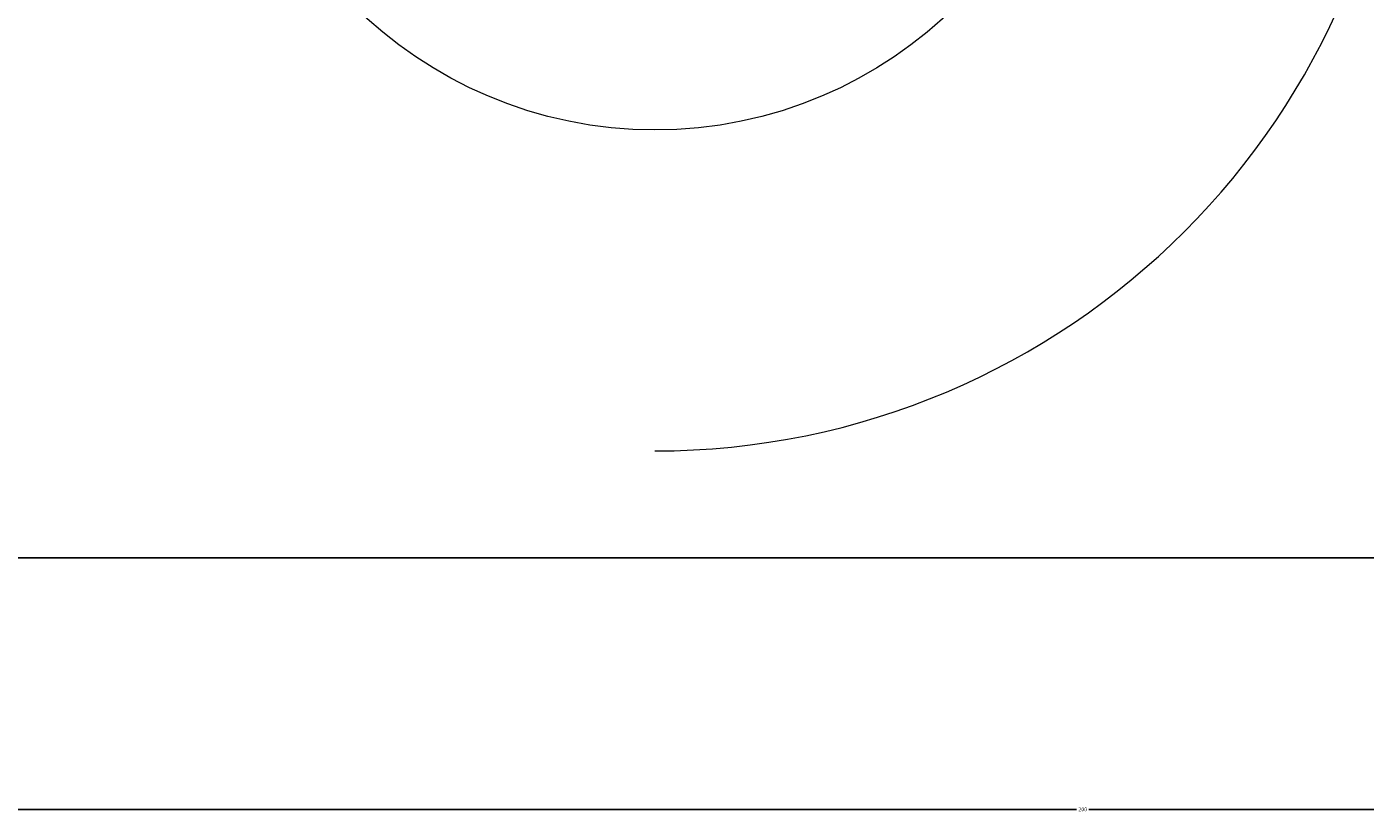
# Model space of a CAD drawing. Units: millimetres. Extents: x 3108 to 3332, y 1482 to 1586.
# Tile 2 of 5: x 3171 to 3233, y 1482 to 1519. Entities that reach past the tile are written whole.
import ezdxf

# ---------------------------------------------------------------- set-up
doc = ezdxf.new("R2010")
doc.units = ezdxf.units.MM
doc.layers.add('M-CONS', color=8, linetype='Continuous', lineweight=18)
doc.layers.add('M-DIMS', color=2, linetype='Continuous', lineweight=18)
doc.styles.get("Standard").update_dxf_attribs({"font": 'arial.ttf'})
doc.dimstyles.get("Standard").update_dxf_attribs({"dimtxt": 0.18, "dimasz": 0.18, "dimexe": 0.18, "dimexo": 0.0625, "dimgap": 0.09, "dimtad": 0, "dimtih": 1, "dimtoh": 1, "dimdec": 4, "dimzin": 0, "dimdsep": 46, "dimtxsty": 'Standard', "dimcen": 0.09, "dimadec": 0, "dimazin": 0, "dimtfac": 1, "dimtdec": 4, "dimtofl": 0, "dimtmove": 0, "dimatfit": 3, "dimfxl": 1, "dimtolj": 1, "dimtzin": 0, "dimarcsym": 0})

# ---------------------------------------------------------------- blocks, each defined once
blk = doc.blocks.new('*D1')
at = {"layer": 'Defpoints', "color": 0, "transparency": 16777216}
for p in [(3119.945, 1498.943), (3319.945, 1493.943), (3319.945, 1482.193)]:
    blk.add_point(p, dxfattribs=at)
at = {"layer": 'M-DIMS', "color": 0, "lineweight": -2, "transparency": 16777216}
for p, q in [((3119.945, 1498.881), (3119.945, 1482.013)), ((3319.945, 1493.881), (3319.945, 1482.013)), ((3120.125, 1482.193), (3219.655, 1482.193)), ((3319.765, 1482.193), (3220.235, 1482.193))]:
    blk.add_line(p, q, dxfattribs=at)
at = {"layer": 'M-DIMS', "color": 0, "transparency": 16777216}
for points in [[(3120.125, 1482.223), (3120.125, 1482.163), (3119.945, 1482.193)], [(3319.765, 1482.223), (3319.765, 1482.163), (3319.945, 1482.193)]]:
    blk.add_solid(points, dxfattribs=at)
at = {"layer": 'M-DIMS', "color": 0, "transparency": 16777216, "insert": (3219.945, 1482.193), "char_height": 0.18, "attachment_point": 5}
blk.add_mtext('\\A1;200', dxfattribs=at)
blk = doc.blocks.new('*D9')
at = {"layer": 'Defpoints', "color": 0, "transparency": 16777216}
for p in [(3108.195, 1533.943), (3199.945, 1533.943), (3159.945, 1498.943)]:
    blk.add_point(p, dxfattribs=at)
at = {"layer": 'M-DIMS', "color": 0, "lineweight": -2, "transparency": 16777216}
for p, q in [((3199.882, 1533.943), (3108.015, 1533.943)), ((3108.195, 1533.763), (3108.195, 1516.625)), ((3108.195, 1499.123), (3108.195, 1516.261)), ((3159.882, 1498.943), (3108.015, 1498.943))]:
    blk.add_line(p, q, dxfattribs=at)
at = {"layer": 'M-DIMS', "color": 0, "transparency": 16777216}
for points in [[(3108.165, 1533.763), (3108.225, 1533.763), (3108.195, 1533.943)], [(3108.165, 1499.123), (3108.225, 1499.123), (3108.195, 1498.943)]]:
    blk.add_solid(points, dxfattribs=at)
at = {"layer": 'M-DIMS', "color": 0, "transparency": 16777216, "insert": (3108.195, 1516.443), "char_height": 0.18, "attachment_point": 5}
blk.add_mtext('\\A1;35', dxfattribs=at)
blk = doc.blocks.new('*D10')
at = {"layer": 'Defpoints', "color": 0, "transparency": 16777216}
for p in [(3119.945, 1498.943), (3108.195, 1493.943), (3319.945, 1493.943)]:
    blk.add_point(p, dxfattribs=at)
at = {"layer": 'M-DIMS', "color": 0, "lineweight": -2, "transparency": 16777216}
for p, q in [((3119.882, 1498.943), (3108.015, 1498.943)), ((3108.195, 1498.763), (3108.195, 1496.625)), ((3108.195, 1494.123), (3108.195, 1496.262)), ((3319.882, 1493.943), (3108.015, 1493.943))]:
    blk.add_line(p, q, dxfattribs=at)
at = {"layer": 'M-DIMS', "color": 0, "transparency": 16777216}
for points in [[(3108.165, 1498.763), (3108.225, 1498.763), (3108.195, 1498.943)], [(3108.165, 1494.123), (3108.225, 1494.123), (3108.195, 1493.943)]]:
    blk.add_solid(points, dxfattribs=at)
at = {"layer": 'M-DIMS', "color": 0, "transparency": 16777216, "insert": (3108.195, 1496.443), "char_height": 0.18, "attachment_point": 5}
blk.add_mtext('\\A1;5', dxfattribs=at)

msp = doc.modelspace()

# ---------------------------------------------------------------- linework, layer by layer
at = {"layer": 'M-CONS'}
msp.add_circle((3199.9448, 1533.9431), 20, dxfattribs=at)
msp.add_arc((3199.9448, 1533.9431), 35, 270, 90, dxfattribs=at)

# ---------------------------------------------------------------- dimensions: what is measured, and where the dimension line sits
at = {"layer": 'M-DIMS'}
for base, p1, p2, picture, middle in [((3108.1948, 1533.9431), (3159.9448, 1498.9431), (3199.9448, 1533.9431), '*D9', (3108.1948, 1516.4431)), ((3108.1948, 1493.9431), (3119.9448, 1498.9431), (3319.9448, 1493.9431), '*D10', (3108.1948, 1496.4431))]:
    dim = msp.add_linear_dim(base=base, p1=p1, p2=p2, angle=90, dimstyle='Standard', override={"dimdec": 0, "dimlfac": 1, "dimrnd": 0, "dimzin": 0, "dimdsep": 46, "dimlunit": 2}, dxfattribs=at)
    dim.commit()
    dim.dimension.update_dxf_attribs({"geometry": picture, "text_midpoint": middle})
dim = msp.add_linear_dim(base=(3319.9448, 1482.1931), p1=(3119.9448, 1498.9431), p2=(3319.9448, 1493.9431), dimstyle='Standard', override={"dimdec": 0, "dimlfac": 1, "dimrnd": 0, "dimzin": 0, "dimdsep": 46, "dimlunit": 2}, dxfattribs=at)
dim.commit()
dim.dimension.update_dxf_attribs({"geometry": '*D1', "text_midpoint": (3219.9448, 1482.1931)})

doc.saveas('drawing.dxf')
